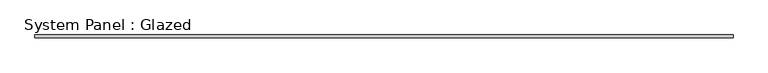
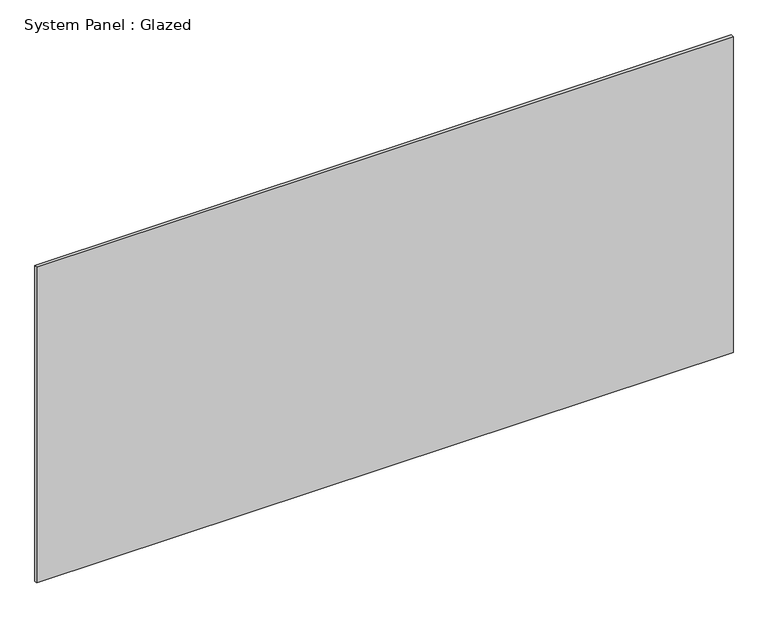
"""IFC4 building model written with IfcOpenShell, lengths in millimetres: plate geometry, System Panel : Glazed."""

from ifc_helpers import new_model, si_unit, origin, origin_with_axes, place, context, project, spatial, polyline, outline, extrude, source, transform, mapped, element, save


def system_panel_glazed_8d480110(model_context):
    return source(origin(), model_context, "Body", "SweptSolid", [
        extrude(outline(polyline([(3175.0, 19.05), (-3175.0, 19.05), (-3175.0, 44.45), (3175.0, 44.45), (3175.0, 19.05)])), origin_with_axes(), (0.0, 0.0, 1.0), 3048.0),
    ])


if __name__ == "__main__":
    model = new_model("IFC4")
    model_context = context("Model", 3, world=origin())
    ifc_project = project(units=[si_unit("LENGTHUNIT", "METRE", prefix="MILLI")], contexts=[model_context])
    site = spatial("IfcSite", under=ifc_project)
    building = spatial("IfcBuilding", under=site)
    placement = place(None, origin())
    system_panel_glazed_shape = system_panel_glazed_8d480110(model_context)
    element("IfcPlate", 1, ObjectType="System Panel : Glazed", at=placement, inside=building, context=model_context, shape_type="MappedRepresentation", body=[
        mapped(system_panel_glazed_shape, transform((0.0, 0.0, 0.0), x_axis=(1.0, 0.0, 0.0), y_axis=(0.0, 1.0, 0.0), z_axis=(0.0, 0.0, 1.0))),
    ])
    save(model, "model.ifc")

# Revit data of these elements
# Type "System Panel : Glazed"
#   Construction Type Id = "GSP4R"
#   Analytic Construction = "1/8 in Pilkington single glazing"
#   Visual Light Transmittance = 0.9
#   Solar Heat Gain Coefficient = 0.86
#   Heat Transfer Coefficient (U) = 1.18115 BTU/(h·ft²·°F)
# Element 1 (IfcPlate, "System Panel : Glazed")
#   Materials on its faces: "Glass"
# Materials
#   "Glass": class "Glass", colour RGB 0 128 192, transparency 0.75, Description = "Soda Lime Glass", Cost = 0
